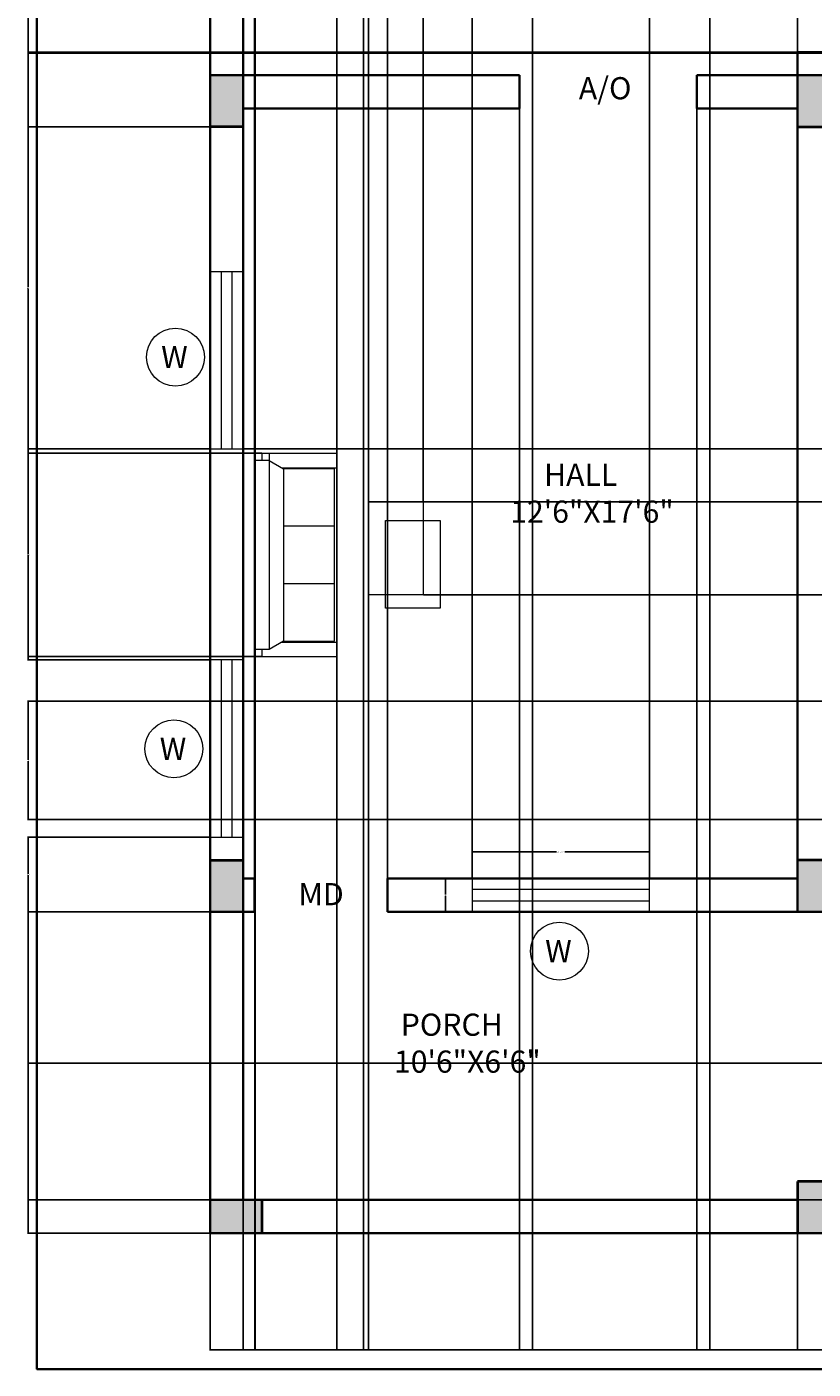
# Model space of a CAD drawing. Units: inches. Extents: x 2243 to 2668, y 14541 to 15226.
# Tile 1 of 5: x 2243 to 2456, y 14541 to 14904. Entities that reach past the tile are written whole.
import ezdxf

# ---------------------------------------------------------------- set-up
doc = ezdxf.new("R2010")
doc.units = ezdxf.units.IN
doc.header["$MEASUREMENT"] = 0
for name, color, linetype, lineweight in [('A-ANNO-DIMS', 2, 'Continuous', 18), ('A-ANNO-SYMB', 3, 'Continuous', 18), ('A-ANNO-TTLB', 7, 'Continuous', 35), ('A-AREA-IDEN', 7, 'Continuous', 18), ('A-COLS', 7, 'Continuous', 40), ('A-COLS-PATT', 7, 'Continuous', 13), ('A-FURN', 8, 'Continuous', 18), ('A-GLAZ', 4, 'Continuous', 18), ('A-WALL', 7, 'Continuous', 35)]:
    doc.layers.add(name, color=color, linetype=linetype, lineweight=lineweight)
doc.styles.get("Standard").update_dxf_attribs({"font": 'arial.ttf'})
doc.dimstyles.get("Standard").update_dxf_attribs({"dimtxt": 0.18, "dimasz": 0.18, "dimexe": 0.18, "dimexo": 0.0625, "dimgap": 0.09, "dimtad": 0, "dimtih": 1, "dimtoh": 1, "dimdec": 4, "dimzin": 0, "dimdsep": 46, "dimtxsty": 'Standard', "dimcen": 0.09, "dimadec": 0, "dimazin": 0, "dimtfac": 1, "dimtdec": 4, "dimtofl": 0, "dimtmove": 0, "dimatfit": 3, "dimfxl": 1, "dimtolj": 1, "dimtzin": 0, "dimarcsym": 0})

# ---------------------------------------------------------------- blocks, each defined once
blk = doc.blocks.new('WIN-48IN')
for p, q in [((0, 9), (0, 0)), ((48, 9), (0, 9)), ((48, 0), (48, 9)), ((48, 6), (0, 6)), ((0, 3), (48, 3)), ((0, 0), (48, 0))]:
    blk.add_line(p, q)
blk = doc.blocks.new('TAG-WINDOW-W')
blk.add_circle((7.84, 7.84), 7.84)
at = {"insert": (3.99, 10.84), "char_height": 6, "attachment_point": 1}
blk.add_mtext_dynamic_manual_height_columns('W', width=14.3449, gutter_width=30, heights=[0], dxfattribs=at)
blk = doc.blocks.new('*D7')
at = {"layer": 'A-ANNO-DIMS', "color": 0, "lineweight": -2, "transparency": 16777216}
for p, q in [((2363.89, 14673.7), (2363.89, 14681.02)), ((2364.07, 14680.84), (2386.77, 14680.84)), ((2411.71, 14680.84), (2389.01, 14680.84)), ((2411.89, 14673.7), (2411.89, 14681.02))]:
    blk.add_line(p, q, dxfattribs=at)
at = {"layer": 'A-ANNO-DIMS', "color": 0, "transparency": 16777216}
for points in [[(2364.07, 14680.87), (2364.07, 14680.81), (2363.89, 14680.84)], [(2411.71, 14680.87), (2411.71, 14680.81), (2411.89, 14680.84)]]:
    blk.add_solid(points, dxfattribs=at)
at = {"layer": 'Defpoints', "color": 0, "transparency": 16777216}
for p in [(2363.89, 14680.84), (2363.89, 14673.64), (2411.89, 14673.64)]:
    blk.add_point(p, dxfattribs=at)
at = {"layer": 'A-ANNO-DIMS', "color": 0, "transparency": 16777216, "insert": (2387.89, 14680.84), "char_height": 0.18, "attachment_point": 5}
blk.add_mtext('\\A1;WINDOW 48 TYP.', dxfattribs=at)
blk = doc.blocks.new('*D8')
at = {"layer": 'A-ANNO-DIMS', "color": 0, "lineweight": -2, "transparency": 16777216}
for p, q in [((2363.83, 14673.64), (2356.51, 14673.64)), ((2356.69, 14673.46), (2356.69, 14669.32)), ((2356.69, 14664.82), (2356.69, 14668.95)), ((2363.83, 14664.64), (2356.51, 14664.64))]:
    blk.add_line(p, q, dxfattribs=at)
at = {"layer": 'A-ANNO-DIMS', "color": 0, "transparency": 16777216}
for points in [[(2356.66, 14673.46), (2356.72, 14673.46), (2356.69, 14673.64)], [(2356.66, 14664.82), (2356.72, 14664.82), (2356.69, 14664.64)]]:
    blk.add_solid(points, dxfattribs=at)
at = {"layer": 'Defpoints', "color": 0, "transparency": 16777216}
for p in [(2363.89, 14673.64), (2356.69, 14664.64), (2363.89, 14664.64)]:
    blk.add_point(p, dxfattribs=at)
at = {"layer": 'A-ANNO-DIMS', "color": 0, "transparency": 16777216, "insert": (2356.69, 14669.14), "char_height": 0.18, "attachment_point": 5}
blk.add_mtext('\\A1;9 TYP.', dxfattribs=at)
blk = doc.blocks.new('*D19')
at = {"layer": 'A-ANNO-DIMS', "color": 0, "lineweight": -2, "transparency": 16777216}
for p, q in [((2292.96, 14577.57), (2292.96, 14545.86)), ((2451.96, 14577.57), (2451.96, 14545.86)), ((2293.14, 14546.04), (2372.18, 14546.04)), ((2451.78, 14546.04), (2372.74, 14546.04))]:
    blk.add_line(p, q, dxfattribs=at)
at = {"layer": 'A-ANNO-DIMS', "color": 0, "transparency": 16777216}
for points in [[(2293.14, 14546.07), (2293.14, 14546.01), (2292.96, 14546.04)], [(2451.78, 14546.07), (2451.78, 14546.01), (2451.96, 14546.04)]]:
    blk.add_solid(points, dxfattribs=at)
at = {"layer": 'Defpoints', "color": 0, "transparency": 16777216}
for p in [(2292.96, 14577.64), (2451.96, 14577.64), (2451.96, 14546.04)]:
    blk.add_point(p, dxfattribs=at)
at = {"layer": 'A-ANNO-DIMS', "color": 0, "transparency": 16777216, "insert": (2372.46, 14546.04), "char_height": 0.18, "attachment_point": 5}
blk.add_mtext('\\A1;159', dxfattribs=at)
blk = doc.blocks.new('*D20')
at = {"layer": 'A-ANNO-DIMS', "color": 0, "lineweight": -2, "transparency": 16777216}
for p, q in [((2451.96, 14577.57), (2451.96, 14545.86)), ((2604.96, 14577.57), (2604.96, 14545.86)), ((2452.14, 14546.04), (2528.18, 14546.04)), ((2604.78, 14546.04), (2528.74, 14546.04))]:
    blk.add_line(p, q, dxfattribs=at)
at = {"layer": 'A-ANNO-DIMS', "color": 0, "transparency": 16777216}
for points in [[(2452.14, 14546.07), (2452.14, 14546.01), (2451.96, 14546.04)], [(2604.78, 14546.07), (2604.78, 14546.01), (2604.96, 14546.04)]]:
    blk.add_solid(points, dxfattribs=at)
at = {"layer": 'Defpoints', "color": 0, "transparency": 16777216}
for p in [(2451.96, 14577.64), (2604.96, 14577.64), (2604.96, 14546.04)]:
    blk.add_point(p, dxfattribs=at)
at = {"layer": 'A-ANNO-DIMS', "color": 0, "transparency": 16777216, "insert": (2528.46, 14546.04), "char_height": 0.18, "attachment_point": 5}
blk.add_mtext('\\A1;153', dxfattribs=at)
blk = doc.blocks.new('*D21')
at = {"layer": 'A-ANNO-DIMS', "color": 0, "lineweight": -2, "transparency": 16777216}
for p, q in [((2292.9, 14664.64), (2243.57, 14664.64)), ((2243.75, 14664.46), (2243.75, 14621.32)), ((2243.75, 14577.82), (2243.75, 14620.95)), ((2292.9, 14577.64), (2243.57, 14577.64))]:
    blk.add_line(p, q, dxfattribs=at)
at = {"layer": 'A-ANNO-DIMS', "color": 0, "transparency": 16777216}
for points in [[(2243.72, 14664.46), (2243.78, 14664.46), (2243.75, 14664.64)], [(2243.72, 14577.82), (2243.78, 14577.82), (2243.75, 14577.64)]]:
    blk.add_solid(points, dxfattribs=at)
at = {"layer": 'Defpoints', "color": 0, "transparency": 16777216}
for p in [(2243.75, 14664.64), (2292.96, 14664.64), (2292.96, 14577.64)]:
    blk.add_point(p, dxfattribs=at)
at = {"layer": 'A-ANNO-DIMS', "color": 0, "transparency": 16777216, "insert": (2243.75, 14621.14), "char_height": 0.18, "attachment_point": 5}
blk.add_mtext('\\A1;87', dxfattribs=at)
blk = doc.blocks.new('*D22')
at = {"layer": 'A-ANNO-DIMS', "color": 0, "lineweight": -2, "transparency": 16777216}
for p, q in [((2292.9, 14684.86), (2243.57, 14684.86)), ((2243.75, 14684.68), (2243.75, 14674.93)), ((2243.75, 14664.82), (2243.75, 14674.57)), ((2292.9, 14664.64), (2243.57, 14664.64))]:
    blk.add_line(p, q, dxfattribs=at)
at = {"layer": 'A-ANNO-DIMS', "color": 0, "transparency": 16777216}
for points in [[(2243.72, 14684.68), (2243.78, 14684.68), (2243.75, 14684.86)], [(2243.72, 14664.82), (2243.78, 14664.82), (2243.75, 14664.64)]]:
    blk.add_solid(points, dxfattribs=at)
at = {"layer": 'Defpoints', "color": 0, "transparency": 16777216}
for p in [(2243.75, 14684.86), (2292.96, 14684.86), (2292.96, 14664.64)]:
    blk.add_point(p, dxfattribs=at)
at = {"layer": 'A-ANNO-DIMS', "color": 0, "transparency": 16777216, "insert": (2243.75, 14674.75), "char_height": 0.18, "attachment_point": 5}
blk.add_mtext('\\A1;20.225', dxfattribs=at)
blk = doc.blocks.new('*D23')
at = {"layer": 'A-ANNO-DIMS', "color": 0, "lineweight": -2, "transparency": 16777216}
for p, q in [((2292.9, 14789.95), (2243.57, 14789.95)), ((2243.75, 14789.77), (2243.75, 14761.59)), ((2243.75, 14733.04), (2243.75, 14761.22)), ((2292.9, 14732.86), (2243.57, 14732.86))]:
    blk.add_line(p, q, dxfattribs=at)
at = {"layer": 'A-ANNO-DIMS', "color": 0, "transparency": 16777216}
for points in [[(2243.72, 14789.77), (2243.78, 14789.77), (2243.75, 14789.95)], [(2243.72, 14733.04), (2243.78, 14733.04), (2243.75, 14732.86)]]:
    blk.add_solid(points, dxfattribs=at)
at = {"layer": 'Defpoints', "color": 0, "transparency": 16777216}
for p in [(2243.75, 14789.95), (2292.96, 14789.95), (2292.96, 14732.86)]:
    blk.add_point(p, dxfattribs=at)
at = {"layer": 'A-ANNO-DIMS', "color": 0, "transparency": 16777216, "insert": (2243.75, 14761.41), "char_height": 0.18, "attachment_point": 5}
blk.add_mtext('\\A1;57.09', dxfattribs=at)
blk = doc.blocks.new('*D24')
at = {"layer": 'A-ANNO-DIMS', "color": 0, "lineweight": -2, "transparency": 16777216}
for p, q in [((2292.9, 14877.14), (2243.57, 14877.14)), ((2243.75, 14876.96), (2243.75, 14833.73)), ((2243.75, 14790.13), (2243.75, 14833.36)), ((2292.9, 14789.95), (2243.57, 14789.95))]:
    blk.add_line(p, q, dxfattribs=at)
at = {"layer": 'A-ANNO-DIMS', "color": 0, "transparency": 16777216}
for points in [[(2243.72, 14876.96), (2243.78, 14876.96), (2243.75, 14877.14)], [(2243.72, 14790.13), (2243.78, 14790.13), (2243.75, 14789.95)]]:
    blk.add_solid(points, dxfattribs=at)
at = {"layer": 'Defpoints', "color": 0, "transparency": 16777216}
for p in [(2243.75, 14877.14), (2292.96, 14877.14), (2292.96, 14789.95)]:
    blk.add_point(p, dxfattribs=at)
at = {"layer": 'A-ANNO-DIMS', "color": 0, "transparency": 16777216, "insert": (2243.75, 14833.54), "char_height": 0.18, "attachment_point": 5}
blk.add_mtext('\\A1;87.19', dxfattribs=at)
blk = doc.blocks.new('*D25')
at = {"layer": 'A-ANNO-DIMS', "color": 0, "lineweight": -2, "transparency": 16777216}
for p, q in [((2292.9, 14940.64), (2243.57, 14940.64)), ((2243.75, 14940.46), (2243.75, 14909.07)), ((2243.75, 14877.32), (2243.75, 14908.71)), ((2292.9, 14877.14), (2243.57, 14877.14))]:
    blk.add_line(p, q, dxfattribs=at)
at = {"layer": 'A-ANNO-DIMS', "color": 0, "transparency": 16777216}
for points in [[(2243.72, 14940.46), (2243.78, 14940.46), (2243.75, 14940.64)], [(2243.72, 14877.32), (2243.78, 14877.32), (2243.75, 14877.14)]]:
    blk.add_solid(points, dxfattribs=at)
at = {"layer": 'Defpoints', "color": 0, "transparency": 16777216}
for p in [(2243.75, 14940.64), (2292.96, 14940.64), (2292.96, 14877.14)]:
    blk.add_point(p, dxfattribs=at)
at = {"layer": 'A-ANNO-DIMS', "color": 0, "transparency": 16777216, "insert": (2243.75, 14908.89), "char_height": 0.18, "attachment_point": 5}
blk.add_mtext('\\A1;63.5', dxfattribs=at)
blk = doc.blocks.new('*D32')
at = {"layer": 'A-ANNO-DIMS', "color": 0, "lineweight": -2, "transparency": 16777216}
for p, q in [((2301.96, 14673.7), (2301.96, 15225.04)), ((2302.14, 15224.86), (2303.31, 15224.86)), ((2304.78, 15224.86), (2303.61, 15224.86)), ((2304.96, 14673.7), (2304.96, 15225.04))]:
    blk.add_line(p, q, dxfattribs=at)
at = {"layer": 'A-ANNO-DIMS', "color": 0, "transparency": 16777216}
for points in [[(2302.14, 15224.89), (2302.14, 15224.83), (2301.96, 15224.86)], [(2304.78, 15224.89), (2304.78, 15224.83), (2304.96, 15224.86)]]:
    blk.add_solid(points, dxfattribs=at)
at = {"layer": 'Defpoints', "color": 0, "transparency": 16777216}
for p in [(2304.96, 15224.86), (2301.96, 14673.64), (2304.96, 14673.64)]:
    blk.add_point(p, dxfattribs=at)
at = {"layer": 'A-ANNO-DIMS', "color": 0, "transparency": 16777216, "insert": (2303.46, 15224.86), "char_height": 0.18, "attachment_point": 5}
blk.add_mtext('\\A1;3', dxfattribs=at)
blk = doc.blocks.new('*D33')
at = {"layer": 'A-ANNO-DIMS', "color": 0, "lineweight": -2, "transparency": 16777216}
for p, q in [((2304.96, 14673.7), (2304.96, 15225.04)), ((2305.14, 15224.86), (2322.74, 15224.86)), ((2340.78, 15224.86), (2323.18, 15224.86)), ((2340.96, 14673.7), (2340.96, 15225.04))]:
    blk.add_line(p, q, dxfattribs=at)
at = {"layer": 'A-ANNO-DIMS', "color": 0, "transparency": 16777216}
for points in [[(2305.14, 15224.89), (2305.14, 15224.83), (2304.96, 15224.86)], [(2340.78, 15224.89), (2340.78, 15224.83), (2340.96, 15224.86)]]:
    blk.add_solid(points, dxfattribs=at)
at = {"layer": 'Defpoints', "color": 0, "transparency": 16777216}
for p in [(2340.96, 15224.86), (2304.96, 14673.64), (2340.96, 14673.64)]:
    blk.add_point(p, dxfattribs=at)
at = {"layer": 'A-ANNO-DIMS', "color": 0, "transparency": 16777216, "insert": (2322.96, 15224.86), "char_height": 0.18, "attachment_point": 5}
blk.add_mtext('\\A1;36', dxfattribs=at)
blk = doc.blocks.new('*D34')
at = {"layer": 'A-ANNO-DIMS', "color": 0, "lineweight": -2, "transparency": 16777216}
for p, q in [((2340.96, 14673.7), (2340.96, 15225.04)), ((2341.14, 15224.86), (2352.03, 15224.86)), ((2363.71, 15224.86), (2352.82, 15224.86)), ((2363.89, 14673.7), (2363.89, 15225.04))]:
    blk.add_line(p, q, dxfattribs=at)
at = {"layer": 'A-ANNO-DIMS', "color": 0, "transparency": 16777216}
for points in [[(2341.14, 15224.89), (2341.14, 15224.83), (2340.96, 15224.86)], [(2363.71, 15224.89), (2363.71, 15224.83), (2363.89, 15224.86)]]:
    blk.add_solid(points, dxfattribs=at)
at = {"layer": 'Defpoints', "color": 0, "transparency": 16777216}
for p in [(2363.89, 15224.86), (2340.96, 14673.64), (2363.89, 14673.64)]:
    blk.add_point(p, dxfattribs=at)
at = {"layer": 'A-ANNO-DIMS', "color": 0, "transparency": 16777216, "insert": (2352.43, 15224.86), "char_height": 0.18, "attachment_point": 5}
blk.add_mtext('\\A1;22.93', dxfattribs=at)
blk = doc.blocks.new('*D35')
at = {"layer": 'A-ANNO-DIMS', "color": 0, "lineweight": -2, "transparency": 16777216}
for p, q in [((2411.89, 14673.7), (2411.89, 15225.04)), ((2412.07, 15224.86), (2431.53, 15224.86)), ((2451.78, 15224.86), (2432.32, 15224.86)), ((2451.96, 14673.7), (2451.96, 15225.04))]:
    blk.add_line(p, q, dxfattribs=at)
at = {"layer": 'A-ANNO-DIMS', "color": 0, "transparency": 16777216}
for points in [[(2412.07, 15224.89), (2412.07, 15224.83), (2411.89, 15224.86)], [(2451.78, 15224.89), (2451.78, 15224.83), (2451.96, 15224.86)]]:
    blk.add_solid(points, dxfattribs=at)
at = {"layer": 'Defpoints', "color": 0, "transparency": 16777216}
for p in [(2451.96, 15224.86), (2411.89, 14673.64), (2451.96, 14673.64)]:
    blk.add_point(p, dxfattribs=at)
at = {"layer": 'A-ANNO-DIMS', "color": 0, "transparency": 16777216, "insert": (2431.93, 15224.86), "char_height": 0.18, "attachment_point": 5}
blk.add_mtext('\\A1;40.07', dxfattribs=at)
blk = doc.blocks.new('*D38')
at = {"layer": 'A-ANNO-DIMS', "color": 0, "lineweight": -2, "transparency": 16777216}
for p, q in [((2463.9, 14623.64), (2243.57, 14623.64)), ((2243.75, 14623.46), (2243.75, 14605.32)), ((2243.75, 14586.82), (2243.75, 14604.95)), ((2463.9, 14586.64), (2243.57, 14586.64))]:
    blk.add_line(p, q, dxfattribs=at)
at = {"layer": 'A-ANNO-DIMS', "color": 0, "transparency": 16777216}
for points in [[(2243.72, 14623.46), (2243.78, 14623.46), (2243.75, 14623.64)], [(2243.72, 14586.82), (2243.78, 14586.82), (2243.75, 14586.64)]]:
    blk.add_solid(points, dxfattribs=at)
at = {"layer": 'Defpoints', "color": 0, "transparency": 16777216}
for p in [(2243.75, 14623.64), (2463.96, 14623.64), (2463.96, 14586.64)]:
    blk.add_point(p, dxfattribs=at)
at = {"layer": 'A-ANNO-DIMS', "color": 0, "transparency": 16777216, "insert": (2243.75, 14605.14), "char_height": 0.18, "attachment_point": 5}
blk.add_mtext('\\A1;37', dxfattribs=at)
blk = doc.blocks.new('*D42')
at = {"layer": 'A-ANNO-DIMS', "color": 0, "lineweight": -2, "transparency": 16777216}
for p, q in [((2380.28, 15014.07), (2380.28, 14545.86)), ((2428.28, 15014.07), (2428.28, 14545.86)), ((2380.46, 14546.04), (2404.06, 14546.04)), ((2428.1, 14546.04), (2404.5, 14546.04))]:
    blk.add_line(p, q, dxfattribs=at)
at = {"layer": 'A-ANNO-DIMS', "color": 0, "transparency": 16777216}
for points in [[(2380.46, 14546.07), (2380.46, 14546.01), (2380.28, 14546.04)], [(2428.1, 14546.07), (2428.1, 14546.01), (2428.28, 14546.04)]]:
    blk.add_solid(points, dxfattribs=at)
at = {"layer": 'Defpoints', "color": 0, "transparency": 16777216}
for p in [(2380.28, 15014.14), (2428.28, 15014.14), (2428.28, 14546.04)]:
    blk.add_point(p, dxfattribs=at)
at = {"layer": 'A-ANNO-DIMS', "color": 0, "transparency": 16777216, "insert": (2404.28, 14546.04), "char_height": 0.18, "attachment_point": 5}
blk.add_mtext('\\A1;48', dxfattribs=at)
blk = doc.blocks.new('*D43')
at = {"layer": 'A-ANNO-DIMS', "color": 0, "lineweight": -2, "transparency": 16777216}
for p, q in [((2301.96, 15023.07), (2301.96, 14545.86)), ((2334.46, 15023.07), (2334.46, 14545.86)), ((2302.14, 14546.04), (2317.89, 14546.04)), ((2334.28, 14546.04), (2318.54, 14546.04))]:
    blk.add_line(p, q, dxfattribs=at)
at = {"layer": 'A-ANNO-DIMS', "color": 0, "transparency": 16777216}
for points in [[(2302.14, 14546.07), (2302.14, 14546.01), (2301.96, 14546.04)], [(2334.28, 14546.07), (2334.28, 14546.01), (2334.46, 14546.04)]]:
    blk.add_solid(points, dxfattribs=at)
at = {"layer": 'Defpoints', "color": 0, "transparency": 16777216}
for p in [(2301.96, 15023.14), (2334.46, 15023.14), (2334.46, 14546.04)]:
    blk.add_point(p, dxfattribs=at)
at = {"layer": 'A-ANNO-DIMS', "color": 0, "transparency": 16777216, "insert": (2318.21, 14546.04), "char_height": 0.18, "attachment_point": 5}
blk.add_mtext('\\A1;32.5', dxfattribs=at)
blk = doc.blocks.new('*D47')
at = {"layer": 'A-ANNO-DIMS', "color": 0, "lineweight": -2, "transparency": 16777216}
for p, q in [((2376.7, 14882.07), (2376.7, 14545.86)), ((2424.7, 14882.07), (2424.7, 14545.86)), ((2376.88, 14546.04), (2400.48, 14546.04)), ((2424.52, 14546.04), (2400.92, 14546.04))]:
    blk.add_line(p, q, dxfattribs=at)
at = {"layer": 'A-ANNO-DIMS', "color": 0, "transparency": 16777216}
for points in [[(2376.88, 14546.07), (2376.88, 14546.01), (2376.7, 14546.04)], [(2424.52, 14546.07), (2424.52, 14546.01), (2424.7, 14546.04)]]:
    blk.add_solid(points, dxfattribs=at)
at = {"layer": 'Defpoints', "color": 0, "transparency": 16777216}
for p in [(2376.7, 14882.14), (2424.7, 14882.14), (2424.7, 14546.04)]:
    blk.add_point(p, dxfattribs=at)
at = {"layer": 'A-ANNO-DIMS', "color": 0, "transparency": 16777216, "insert": (2400.7, 14546.04), "char_height": 0.18, "attachment_point": 5}
blk.add_mtext('\\A1;48', dxfattribs=at)
blk = doc.blocks.new('*D50')
at = {"layer": 'A-ANNO-DIMS', "color": 0, "lineweight": -2, "transparency": 16777216}
for p, q in [((2513.4, 14721.64), (2243.57, 14721.64)), ((2243.75, 14721.46), (2243.75, 14705.82)), ((2243.75, 14689.82), (2243.75, 14705.45)), ((2513.4, 14689.64), (2243.57, 14689.64))]:
    blk.add_line(p, q, dxfattribs=at)
at = {"layer": 'A-ANNO-DIMS', "color": 0, "transparency": 16777216}
for points in [[(2243.72, 14721.46), (2243.78, 14721.46), (2243.75, 14721.64)], [(2243.72, 14689.82), (2243.78, 14689.82), (2243.75, 14689.64)]]:
    blk.add_solid(points, dxfattribs=at)
at = {"layer": 'Defpoints', "color": 0, "transparency": 16777216}
for p in [(2243.75, 14721.64), (2513.46, 14721.64), (2513.46, 14689.64)]:
    blk.add_point(p, dxfattribs=at)
at = {"layer": 'A-ANNO-DIMS', "color": 0, "transparency": 16777216, "insert": (2243.75, 14705.64), "char_height": 0.18, "attachment_point": 5}
blk.add_mtext('\\A1;32', dxfattribs=at)
blk = doc.blocks.new('*D51')
at = {"layer": 'A-ANNO-DIMS', "color": 0, "lineweight": -2, "transparency": 16777216}
for p, q in [((2531.4, 14929.14), (2243.57, 14929.14)), ((2243.75, 14928.96), (2243.75, 14913.32)), ((2243.75, 14897.32), (2243.75, 14912.95)), ((2531.4, 14897.14), (2243.57, 14897.14))]:
    blk.add_line(p, q, dxfattribs=at)
at = {"layer": 'A-ANNO-DIMS', "color": 0, "transparency": 16777216}
for points in [[(2243.72, 14928.96), (2243.78, 14928.96), (2243.75, 14929.14)], [(2243.72, 14897.32), (2243.78, 14897.32), (2243.75, 14897.14)]]:
    blk.add_solid(points, dxfattribs=at)
at = {"layer": 'Defpoints', "color": 0, "transparency": 16777216}
for p in [(2243.75, 14929.14), (2531.46, 14929.14), (2531.46, 14897.14)]:
    blk.add_point(p, dxfattribs=at)
at = {"layer": 'A-ANNO-DIMS', "color": 0, "transparency": 16777216, "insert": (2243.75, 14913.14), "char_height": 0.18, "attachment_point": 5}
blk.add_mtext('\\A1;32', dxfattribs=at)
blk = doc.blocks.new('*D54')
at = {"layer": 'A-ANNO-DIMS', "color": 0, "lineweight": -2, "transparency": 16777216}
for p, q in [((2451.9, 14957.21), (2243.57, 14957.21)), ((2243.75, 14957.03), (2243.75, 14927.48)), ((2243.75, 14897.56), (2243.75, 14927.11)), ((2451.9, 14897.38), (2243.57, 14897.38))]:
    blk.add_line(p, q, dxfattribs=at)
at = {"layer": 'A-ANNO-DIMS', "color": 0, "transparency": 16777216}
for points in [[(2243.72, 14957.03), (2243.78, 14957.03), (2243.75, 14957.21)], [(2243.72, 14897.56), (2243.78, 14897.56), (2243.75, 14897.38)]]:
    blk.add_solid(points, dxfattribs=at)
at = {"layer": 'Defpoints', "color": 0, "transparency": 16777216}
for p in [(2243.75, 14957.21), (2451.96, 14957.21), (2451.96, 14897.38)]:
    blk.add_point(p, dxfattribs=at)
at = {"layer": 'A-ANNO-DIMS', "color": 0, "transparency": 16777216, "insert": (2243.75, 14927.3), "char_height": 0.18, "attachment_point": 5}
blk.add_mtext('\\A1;59.83', dxfattribs=at)
blk = doc.blocks.new('*D56')
at = {"layer": 'A-ANNO-DIMS', "color": 0, "lineweight": -2, "transparency": 16777216}
for p, q in [((2305.04, 14786.87), (2305.04, 15225.04)), ((2305.22, 15224.86), (2315.76, 15224.86)), ((2327.09, 15224.86), (2316.55, 15224.86)), ((2327.27, 14788.83), (2327.27, 15225.04))]:
    blk.add_line(p, q, dxfattribs=at)
at = {"layer": 'A-ANNO-DIMS', "color": 0, "transparency": 16777216}
for points in [[(2305.22, 15224.89), (2305.22, 15224.83), (2305.04, 15224.86)], [(2327.09, 15224.89), (2327.09, 15224.83), (2327.27, 15224.86)]]:
    blk.add_solid(points, dxfattribs=at)
at = {"layer": 'Defpoints', "color": 0, "transparency": 16777216}
for p in [(2327.27, 15224.86), (2327.27, 14788.77), (2305.04, 14786.81)]:
    blk.add_point(p, dxfattribs=at)
at = {"layer": 'A-ANNO-DIMS', "color": 0, "transparency": 16777216, "insert": (2316.15, 15224.86), "char_height": 0.18, "attachment_point": 5}
blk.add_mtext('\\A1;22.23', dxfattribs=at)
blk = doc.blocks.new('*D57')
at = {"layer": 'A-ANNO-DIMS', "color": 0, "lineweight": -2, "transparency": 16777216}
for p, q in [((2306.94, 14788.77), (2243.57, 14788.77)), ((2243.75, 14788.59), (2243.75, 14761.43)), ((2243.75, 14733.9), (2243.75, 14761.06)), ((2306.94, 14733.72), (2243.57, 14733.72))]:
    blk.add_line(p, q, dxfattribs=at)
at = {"layer": 'A-ANNO-DIMS', "color": 0, "transparency": 16777216}
for points in [[(2243.72, 14788.59), (2243.78, 14788.59), (2243.75, 14788.77)], [(2243.72, 14733.9), (2243.78, 14733.9), (2243.75, 14733.72)]]:
    blk.add_solid(points, dxfattribs=at)
at = {"layer": 'Defpoints', "color": 0, "transparency": 16777216}
for p in [(2307, 14788.77), (2243.75, 14733.72), (2307, 14733.72)]:
    blk.add_point(p, dxfattribs=at)
at = {"layer": 'A-ANNO-DIMS', "color": 0, "transparency": 16777216, "insert": (2243.75, 14761.24), "char_height": 0.18, "attachment_point": 5}
blk.add_mtext('\\A1;55.04', dxfattribs=at)
blk = doc.blocks.new('*D58')
at = {"layer": 'A-ANNO-DIMS', "color": 0, "lineweight": -2, "transparency": 16777216}
for p, q in [((2327.27, 14788.7), (2327.27, 14545.86)), ((2335.83, 14775.57), (2335.83, 14545.86)), ((2327.45, 14546.04), (2331.15, 14546.04)), ((2335.65, 14546.04), (2331.94, 14546.04))]:
    blk.add_line(p, q, dxfattribs=at)
at = {"layer": 'A-ANNO-DIMS', "color": 0, "transparency": 16777216}
for points in [[(2327.45, 14546.07), (2327.45, 14546.01), (2327.27, 14546.04)], [(2335.65, 14546.07), (2335.65, 14546.01), (2335.83, 14546.04)]]:
    blk.add_solid(points, dxfattribs=at)
at = {"layer": 'Defpoints', "color": 0, "transparency": 16777216}
for p in [(2327.27, 14788.77), (2335.83, 14775.64), (2335.83, 14546.04)]:
    blk.add_point(p, dxfattribs=at)
at = {"layer": 'A-ANNO-DIMS', "color": 0, "transparency": 16777216, "insert": (2331.55, 14546.04), "char_height": 0.18, "attachment_point": 5}
blk.add_mtext('\\A1;8.562', dxfattribs=at)
blk = doc.blocks.new('*D59')
at = {"layer": 'A-ANNO-DIMS', "color": 0, "lineweight": -2, "transparency": 16777216}
for p, q in [((2335.83, 14775.7), (2335.83, 15225.04)), ((2336.01, 15224.86), (2342.78, 15224.86)), ((2350.47, 15224.86), (2343.69, 15224.86)), ((2350.65, 14775.7), (2350.65, 15225.04))]:
    blk.add_line(p, q, dxfattribs=at)
at = {"layer": 'A-ANNO-DIMS', "color": 0, "transparency": 16777216}
for points in [[(2336.01, 15224.89), (2336.01, 15224.83), (2335.83, 15224.86)], [(2350.47, 15224.89), (2350.47, 15224.83), (2350.65, 15224.86)]]:
    blk.add_solid(points, dxfattribs=at)
at = {"layer": 'Defpoints', "color": 0, "transparency": 16777216}
for p in [(2350.65, 15224.86), (2335.83, 14775.64), (2350.65, 14775.64)]:
    blk.add_point(p, dxfattribs=at)
at = {"layer": 'A-ANNO-DIMS', "color": 0, "transparency": 16777216, "insert": (2343.24, 15224.86), "char_height": 0.18, "attachment_point": 5}
blk.add_mtext('\\A1;14.818', dxfattribs=at)
blk = doc.blocks.new('*D60')
at = {"layer": 'A-ANNO-DIMS', "color": 0, "lineweight": -2, "transparency": 16777216}
for p, q in [((2350.71, 14775.64), (2653.58, 14775.64)), ((2653.4, 14775.46), (2653.4, 14763.21)), ((2653.4, 14750.6), (2653.4, 14762.85)), ((2350.71, 14750.42), (2653.58, 14750.42))]:
    blk.add_line(p, q, dxfattribs=at)
at = {"layer": 'A-ANNO-DIMS', "color": 0, "transparency": 16777216}
for points in [[(2653.37, 14775.46), (2653.43, 14775.46), (2653.4, 14775.64)], [(2653.37, 14750.6), (2653.43, 14750.6), (2653.4, 14750.42)]]:
    blk.add_solid(points, dxfattribs=at)
at = {"layer": 'Defpoints', "color": 0, "transparency": 16777216}
for p in [(2350.65, 14775.64), (2653.4, 14775.64), (2350.65, 14750.42)]:
    blk.add_point(p, dxfattribs=at)
at = {"layer": 'A-ANNO-DIMS', "color": 0, "transparency": 16777216, "insert": (2653.4, 14763.03), "char_height": 0.18, "attachment_point": 5}
blk.add_mtext('\\A1;25.22', dxfattribs=at)
blk = doc.blocks.new('*D61')
at = {"layer": 'A-ANNO-DIMS', "color": 0, "lineweight": -2, "transparency": 16777216}
for p, q in [((2301.96, 15023.07), (2301.96, 14545.86)), ((2380.28, 15014.07), (2380.28, 14545.86)), ((2302.14, 14546.04), (2340.73, 14546.04)), ((2380.1, 14546.04), (2341.51, 14546.04))]:
    blk.add_line(p, q, dxfattribs=at)
at = {"layer": 'A-ANNO-DIMS', "color": 0, "transparency": 16777216}
for points in [[(2302.14, 14546.07), (2302.14, 14546.01), (2301.96, 14546.04)], [(2380.1, 14546.07), (2380.1, 14546.01), (2380.28, 14546.04)]]:
    blk.add_solid(points, dxfattribs=at)
at = {"layer": 'Defpoints', "color": 0, "transparency": 16777216}
for p in [(2301.96, 15023.14), (2380.28, 15014.14), (2380.28, 14546.04)]:
    blk.add_point(p, dxfattribs=at)
at = {"layer": 'A-ANNO-DIMS', "color": 0, "transparency": 16777216, "insert": (2341.12, 14546.04), "char_height": 0.18, "attachment_point": 5}
blk.add_mtext('\\A1;78.32', dxfattribs=at)
blk = doc.blocks.new('*D62')
at = {"layer": 'A-ANNO-DIMS', "color": 0, "lineweight": -2, "transparency": 16777216}
for p, q in [((2301.96, 14882.07), (2301.96, 14545.86)), ((2376.7, 14882.07), (2376.7, 14545.86)), ((2302.14, 14546.04), (2338.94, 14546.04)), ((2376.52, 14546.04), (2339.72, 14546.04))]:
    blk.add_line(p, q, dxfattribs=at)
at = {"layer": 'A-ANNO-DIMS', "color": 0, "transparency": 16777216}
for points in [[(2302.14, 14546.07), (2302.14, 14546.01), (2301.96, 14546.04)], [(2376.52, 14546.07), (2376.52, 14546.01), (2376.7, 14546.04)]]:
    blk.add_solid(points, dxfattribs=at)
at = {"layer": 'Defpoints', "color": 0, "transparency": 16777216}
for p in [(2301.96, 14882.14), (2376.7, 14882.14), (2376.7, 14546.04)]:
    blk.add_point(p, dxfattribs=at)
at = {"layer": 'A-ANNO-DIMS', "color": 0, "transparency": 16777216, "insert": (2339.33, 14546.04), "char_height": 0.18, "attachment_point": 5}
blk.add_mtext('\\A1;74.74', dxfattribs=at)
blk = doc.blocks.new('*D63')
at = {"layer": 'A-ANNO-DIMS', "color": 0, "lineweight": -2, "transparency": 16777216}
for p, q in [((2305.04, 14735.62), (2305.04, 14545.86)), ((2301.96, 14732.8), (2301.96, 14545.86)), ((2302.14, 14546.04), (2303.1, 14546.04)), ((2304.86, 14546.04), (2303.89, 14546.04))]:
    blk.add_line(p, q, dxfattribs=at)
at = {"layer": 'A-ANNO-DIMS', "color": 0, "transparency": 16777216}
for points in [[(2302.14, 14546.07), (2302.14, 14546.01), (2301.96, 14546.04)], [(2304.86, 14546.07), (2304.86, 14546.01), (2305.04, 14546.04)]]:
    blk.add_solid(points, dxfattribs=at)
at = {"layer": 'Defpoints', "color": 0, "transparency": 16777216}
for p in [(2305.04, 14735.68), (2301.96, 14732.86), (2305.04, 14546.04)]:
    blk.add_point(p, dxfattribs=at)
at = {"layer": 'A-ANNO-DIMS', "color": 0, "transparency": 16777216, "insert": (2303.5, 14546.04), "char_height": 0.18, "attachment_point": 5}
blk.add_mtext('\\A1;3.077', dxfattribs=at)
blk = doc.blocks.new('*D64')
at = {"layer": 'A-ANNO-DIMS', "color": 0, "lineweight": -2, "transparency": 16777216}
for p, q in [((2302.02, 14789.95), (2653.58, 14789.95)), ((2653.4, 14789.77), (2653.4, 14782.98)), ((2653.4, 14775.82), (2653.4, 14782.61)), ((2335.89, 14775.64), (2653.58, 14775.64))]:
    blk.add_line(p, q, dxfattribs=at)
at = {"layer": 'A-ANNO-DIMS', "color": 0, "transparency": 16777216}
for points in [[(2653.37, 14789.77), (2653.43, 14789.77), (2653.4, 14789.95)], [(2653.37, 14775.82), (2653.43, 14775.82), (2653.4, 14775.64)]]:
    blk.add_solid(points, dxfattribs=at)
at = {"layer": 'Defpoints', "color": 0, "transparency": 16777216}
for p in [(2301.96, 14789.95), (2335.83, 14775.64), (2653.4, 14775.64)]:
    blk.add_point(p, dxfattribs=at)
at = {"layer": 'A-ANNO-DIMS', "color": 0, "transparency": 16777216, "insert": (2653.4, 14782.79), "char_height": 0.18, "attachment_point": 5}
blk.add_mtext('\\A1;14.312', dxfattribs=at)
blk = doc.blocks.new('*D65')
at = {"layer": 'A-ANNO-DIMS', "color": 0, "lineweight": -2, "transparency": 16777216}
for p, q in [((2305.17, 15053.26), (2305.17, 14545.86)), ((2301.96, 15035.22), (2301.96, 14545.86)), ((2302.14, 14546.04), (2303.26, 14546.04)), ((2304.99, 14546.04), (2303.87, 14546.04))]:
    blk.add_line(p, q, dxfattribs=at)
at = {"layer": 'A-ANNO-DIMS', "color": 0, "transparency": 16777216}
for points in [[(2302.14, 14546.07), (2302.14, 14546.01), (2301.96, 14546.04)], [(2304.99, 14546.07), (2304.99, 14546.01), (2305.17, 14546.04)]]:
    blk.add_solid(points, dxfattribs=at)
at = {"layer": 'Defpoints', "color": 0, "transparency": 16777216}
for p in [(2305.17, 15053.32), (2301.96, 15035.28), (2305.17, 14546.04)]:
    blk.add_point(p, dxfattribs=at)
at = {"layer": 'A-ANNO-DIMS', "color": 0, "transparency": 16777216, "insert": (2303.56, 14546.04), "char_height": 0.18, "attachment_point": 5}
blk.add_mtext('\\A1;3.21', dxfattribs=at)

msp = doc.modelspace()

# ---------------------------------------------------------------- hatches: boundary and pattern name
at = {"layer": 'A-COLS-PATT'}
h = msp.add_hatch(color=256, dxfattribs=at)
h.dxf.hatch_style = 1
h.paths.add_polyline_path([(2301.96, 15176.1368), (2292.96, 15176.1368), (2292.96, 15162.1368), (2301.96, 15162.1368)])
h.paths.add_polyline_path([(2460.96, 15176.1368), (2451.96, 15176.1368), (2451.96, 15162.1368), (2460.96, 15162.1368)])
h.paths.add_polyline_path([(2604.96, 15176.1368), (2595.96, 15176.1368), (2595.96, 15162.1368), (2604.96, 15162.1368)])
h.paths.add_polyline_path([(2301.96, 15028.1368), (2292.96, 15028.1368), (2292.96, 15014.1368), (2301.96, 15014.1368)])
h.paths.add_polyline_path([(2460.96, 15028.1368), (2451.96, 15028.1368), (2451.96, 15014.1368), (2460.96, 15014.1368)])
h.paths.add_polyline_path([(2604.96, 15027.8868), (2595.96, 15027.8868), (2595.96, 15013.8868), (2604.96, 15013.8868)])
h.paths.add_polyline_path([(2301.96, 14891.1368), (2292.96, 14891.1368), (2292.96, 14877.1368), (2301.96, 14877.1368)])
h.paths.add_polyline_path([(2460.96, 14891.1368), (2451.96, 14891.1368), (2451.96, 14877.1368), (2460.96, 14877.1368)])
h.paths.add_polyline_path([(2604.96, 14891.1368), (2595.96, 14891.1368), (2595.96, 14877.1368), (2604.96, 14877.1368)])
h.paths.add_polyline_path([(2301.96, 14678.6368), (2292.96, 14678.6368), (2292.96, 14664.6368), (2301.96, 14664.6368)])
h.paths.add_polyline_path([(2460.96, 14678.6368), (2451.96, 14678.6368), (2451.96, 14664.6368), (2460.96, 14664.6368)])
h.paths.add_polyline_path([(2604.96, 14678.6368), (2595.96, 14678.6368), (2595.96, 14664.6368), (2604.96, 14664.6368)])
h.paths.add_polyline_path([(2604.96, 14591.6368), (2595.96, 14591.6368), (2595.96, 14577.6368), (2604.96, 14577.6368)])
h.paths.add_polyline_path([(2460.96, 14591.6368), (2451.96, 14591.6368), (2451.96, 14577.6368), (2460.96, 14577.6368)])
h.paths.add_polyline_path([(2306.96, 14586.6368), (2292.96, 14586.6368), (2292.96, 14577.6368), (2306.96, 14577.6368)])

# ---------------------------------------------------------------- linework, layer by layer
at = {"layer": 'A-ANNO-TTLB'}
msp.add_lwpolyline([(2246.1122, 15225.9536), (2667.5226, 15225.9536), (2667.5226, 14540.814), (2246.1122, 14540.814)], close=True, dxfattribs=at)
at = {"layer": 'A-COLS'}
for p, q in [((2301.96, 14877.1368), (2292.96, 14877.1368)), ((2451.96, 14877.1368), (2460.96, 14877.1368)), ((2292.96, 14678.6368), (2301.96, 14678.6368)), ((2460.96, 14678.6368), (2451.96, 14678.6368)), ((2460.96, 14591.6368), (2451.96, 14591.6368)), ((2451.96, 14591.6368), (2451.96, 14577.6368)), ((2306.96, 14586.6368), (2306.96, 14577.6368))]:
    msp.add_line(p, q, dxfattribs=at)
at = {"layer": 'A-FURN'}
for p, q in [((2306.9985, 14788.7668), (2327.2661, 14788.7668)), ((2306.9985, 14788.7668), (2306.9985, 14786.8054)), ((2308.9599, 14788.7668), (2308.9599, 14735.6842)), ((2327.2661, 14784.844), (2327.2661, 14788.7668)), ((2305.0371, 14786.8054), (2305.0371, 14735.6842)), ((2308.9599, 14786.8054), (2305.0371, 14786.8054)), ((2308.9599, 14786.8054), (2312.8826, 14784.5989)), ((2312.5809, 14784.844), (2327.2661, 14784.844)), ((2326.6123, 14784.5962), (2312.8826, 14784.5962)), ((2326.6123, 14769.0277), (2312.8826, 14769.0277)), ((2326.6123, 14753.4592), (2312.8826, 14753.4592)), ((2312.8826, 14737.8908), (2308.9599, 14735.6842)), ((2312.3222, 14737.6456), (2327.2661, 14737.6456)), ((2327.2661, 14737.6456), (2327.2661, 14733.7228)), ((2308.9599, 14735.6842), (2305.0371, 14735.6842)), ((2306.9985, 14735.6842), (2306.9985, 14733.7228)), ((2306.9985, 14733.7228), (2327.2661, 14733.7228))]:
    msp.add_line(p, q, dxfattribs=at)
msp.add_lwpolyline([(2312.8826, 14784.5989), (2312.8826, 14737.8908), (2326.6123, 14737.8908), (2326.6123, 14784.5962)], dxfattribs=at)
for points in [[(2335.8284, 14775.637), (2350.6465, 14775.637), (2350.6465, 14750.4188), (2335.8284, 14750.4188)], [(2340.4738, 14770.5816), (2355.2919, 14770.5816), (2355.2919, 14746.833), (2340.4738, 14746.833)]]:
    msp.add_lwpolyline(points, close=True, dxfattribs=at)
at = {"layer": 'A-WALL'}
for p, q in [((2292.96, 15176.1368), (2292.96, 14577.6368)), ((2301.96, 15176.1368), (2301.96, 14586.6368)), ((2460.96, 14897.3823), (2451.96, 14897.3823)), ((2451.96, 14897.3823), (2451.96, 14664.6368)), ((2292.96, 14891.1368), (2376.7001, 14891.1368)), ((2376.7001, 14882.1368), (2376.7001, 14891.1368)), ((2424.7001, 14891.1368), (2424.7001, 14882.1368)), ((2424.7001, 14891.1368), (2463.96, 14891.1368)), ((2301.96, 14882.1368), (2376.7001, 14882.1368)), ((2424.7001, 14882.1368), (2451.96, 14882.1368)), ((2301.96, 14673.6368), (2304.96, 14673.6368)), ((2304.96, 14664.6368), (2304.96, 14673.6368)), ((2340.96, 14673.6368), (2340.96, 14664.6368)), ((2340.96, 14673.6368), (2451.96, 14673.6368)), ((2292.96, 14664.6368), (2304.96, 14664.6368)), ((2301.96, 14664.6368), (2304.96, 14664.6368)), ((2340.96, 14664.6368), (2604.96, 14664.6368)), ((2292.96, 14586.6368), (2451.96, 14586.6368)), ((2292.96, 14577.6368), (2604.96, 14577.6368))]:
    msp.add_line(p, q, dxfattribs=at)

# ---------------------------------------------------------------- block references
at = {"layer": 'A-ANNO-SYMB'}
for p in [(2275.7428, 14806.9886), (2275.3529, 14700.9221), (2379.6765, 14646.1627)]:
    msp.add_blockref('TAG-WINDOW-W', p, dxfattribs=at)
at = {"layer": 'A-GLAZ'}
for p, rotation in [((2301.9598, 14789.9494), 89.99999999999363), ((2292.9602, 14732.8617), 269.9999999999944), ((2411.8915, 14673.6366), 180)]:
    msp.add_blockref('WIN-48IN', p, dxfattribs=dict(at, rotation=rotation))

# ---------------------------------------------------------------- texts
at = {"layer": 'A-ANNO-SYMB', "char_height": 6, "attachment_point": 1}
for s, width, insert in [('A/O', 16.844499, (2392.7668, 14890.6173)), ('MD', 13.645752, (2316.8724, 14672.4156))]:
    msp.add_mtext_dynamic_manual_height_columns(s, width=width, gutter_width=30, heights=[0], dxfattribs=dict(at, insert=insert))
at = {"layer": 'A-AREA-IDEN', "char_height": 6, "attachment_point": 1}
for s, width, insert in [('     HALL\\P12\'6"X17\'6"', 53.893278, (2374.2008, 14785.9663)), (' PORCH\\P10\'6"X6\'6"', 72.668828, (2342.7345, 14637.0764))]:
    msp.add_mtext_dynamic_manual_height_columns(s, width=width, gutter_width=30, heights=[0], dxfattribs=dict(at, insert=insert))

# ---------------------------------------------------------------- dimensions: what is measured, and where the dimension line sits
at = {"layer": 'A-ANNO-DIMS'}
for base, p1, p2, override, picture, middle in [((2304.96, 15224.8619), (2301.96, 14673.6368), (2304.96, 14673.6368), {"dimdec": 0, "dimlfac": 1, "dimrnd": 0, "dimzin": 0, "dimdsep": 46, "dimlunit": 2}, '*D32', (2303.46, 15224.8619)), ((2340.96, 15224.8619), (2304.96, 14673.6368), (2340.96, 14673.6368), {"dimdec": 0, "dimlfac": 1, "dimrnd": 0, "dimzin": 0, "dimdsep": 46, "dimlunit": 2}, '*D33', (2322.96, 15224.8619)), ((2327.2661, 15224.8619), (2305.0371, 14786.8054), (2327.2661, 14788.7668), {"dimdec": 2, "dimlfac": 1, "dimrnd": 0, "dimzin": 0, "dimdsep": 46, "dimlunit": 2}, '*D56', (2316.1516, 15224.8619)), ((2350.6465, 15224.8619), (2335.8284, 14775.637), (2350.6465, 14775.637), {"dimdec": 3, "dimlfac": 1, "dimrnd": 0, "dimzin": 0, "dimdsep": 46, "dimlunit": 2}, '*D59', (2343.2375, 15224.8619)), ((2363.8914, 15224.8619), (2340.96, 14673.6368), (2363.8914, 14673.6368), {"dimdec": 2, "dimlfac": 1, "dimrnd": 0, "dimzin": 0, "dimdsep": 46, "dimlunit": 2}, '*D34', (2352.4257, 15224.8619)), ((2451.96, 15224.8619), (2411.8914, 14673.6368), (2451.96, 14673.6368), {"dimdec": 2, "dimlfac": 1, "dimrnd": 0, "dimzin": 0, "dimdsep": 46, "dimlunit": 2}, '*D35', (2431.9257, 15224.8619)), ((2305.1696, 14546.0368), (2301.96, 15035.282), (2305.1696, 15053.321), {"dimdec": 2, "dimlfac": 1, "dimrnd": 0, "dimzin": 0, "dimdsep": 46, "dimlunit": 2}, '*D65', (2303.5648, 14546.0368)), ((2334.4616, 14546.0368), (2301.96, 15023.1368), (2334.4616, 15023.1368), {"dimdec": 1, "dimlfac": 1, "dimrnd": 0, "dimzin": 0, "dimdsep": 46, "dimlunit": 2}, '*D43', (2318.2108, 14546.0368)), ((2380.2818, 14546.0368), (2301.96, 15023.1368), (2380.2818, 15014.1368), {"dimdec": 2, "dimlfac": 1, "dimrnd": 0, "dimzin": 0, "dimdsep": 46, "dimlunit": 2}, '*D61', (2341.1209, 14546.0368)), ((2428.2818, 14546.0368), (2380.2818, 15014.1368), (2428.2818, 15014.1368), {"dimdec": 0, "dimlfac": 1, "dimrnd": 0, "dimzin": 0, "dimdsep": 46, "dimlunit": 2}, '*D42', (2404.2818, 14546.0368)), ((2376.7001, 14546.0368), (2301.96, 14882.1368), (2376.7001, 14882.1368), {"dimdec": 2, "dimlfac": 1, "dimrnd": 0, "dimzin": 0, "dimdsep": 46, "dimlunit": 2}, '*D62', (2339.33, 14546.0368)), ((2424.7001, 14546.0368), (2376.7001, 14882.1368), (2424.7001, 14882.1368), {"dimdec": 0, "dimlfac": 1, "dimrnd": 0, "dimzin": 0, "dimdsep": 46, "dimlunit": 2}, '*D47', (2400.7001, 14546.0368)), ((2335.8284, 14546.0368), (2327.2661, 14788.7668), (2335.8284, 14775.637), {"dimdec": 3, "dimlfac": 1, "dimrnd": 0, "dimzin": 0, "dimdsep": 46, "dimlunit": 2}, '*D58', (2331.5472, 14546.0368)), ((2305.0371, 14546.0368), (2301.96, 14732.8616), (2305.0371, 14735.6842), {"dimdec": 3, "dimlfac": 1, "dimrnd": 0, "dimzin": 0, "dimdsep": 46, "dimlunit": 2}, '*D63', (2303.4985, 14546.0368)), ((2451.96, 14546.0368), (2292.96, 14577.6368), (2451.96, 14577.6368), {"dimdec": 0, "dimlfac": 1, "dimrnd": 0, "dimzin": 0, "dimdsep": 46, "dimlunit": 2}, '*D19', (2372.46, 14546.0368)), ((2604.96, 14546.0368), (2451.96, 14577.6368), (2604.96, 14577.6368), {"dimdec": 0, "dimlfac": 1, "dimrnd": 0, "dimzin": 0, "dimdsep": 46, "dimlunit": 2}, '*D20', (2528.46, 14546.0368))]:
    dim = msp.add_linear_dim(base=base, p1=p1, p2=p2, dimstyle='Standard', override=override, dxfattribs=at)
    dim.commit()
    dim.dimension.update_dxf_attribs({"geometry": picture, "text_midpoint": middle})
for base, p1, p2, override, picture, middle in [((2243.7531, 14957.2115), (2451.96, 14897.3823), (2451.96, 14957.2115), {"dimdec": 2, "dimlfac": 1, "dimrnd": 0, "dimzin": 0, "dimdsep": 46, "dimlunit": 2}, '*D54', (2243.7531, 14927.2969)), ((2243.7531, 14940.6414), (2292.96, 14877.1368), (2292.96, 14940.6414), {"dimdec": 1, "dimlfac": 1, "dimrnd": 0, "dimzin": 0, "dimdsep": 46, "dimlunit": 2}, '*D25', (2243.7531, 14908.8891)), ((2243.7531, 14929.1368), (2531.46, 14897.1368), (2531.46, 14929.1368), {"dimdec": 0, "dimlfac": 1, "dimrnd": 0, "dimzin": 0, "dimdsep": 46, "dimlunit": 2}, '*D51', (2243.7531, 14913.1368)), ((2243.7531, 14877.1368), (2292.96, 14789.9494), (2292.96, 14877.1368), {"dimdec": 2, "dimlfac": 1, "dimrnd": 0, "dimzin": 0, "dimdsep": 46, "dimlunit": 2}, '*D24', (2243.7531, 14833.5431)), ((2243.7531, 14789.9494), (2292.96, 14732.8616), (2292.96, 14789.9494), {"dimdec": 2, "dimlfac": 1, "dimrnd": 0, "dimzin": 0, "dimdsep": 46, "dimlunit": 2}, '*D23', (2243.7531, 14761.4055)), ((2243.7531, 14733.7228), (2306.9985, 14788.7668), (2306.9985, 14733.7228), {"dimdec": 2, "dimlfac": 1, "dimrnd": 0, "dimzin": 0, "dimdsep": 46, "dimlunit": 2}, '*D57', (2243.7531, 14761.2448)), ((2653.4036, 14775.637), (2301.96, 14789.9494), (2335.8284, 14775.637), {"dimdec": 3, "dimlfac": 1, "dimrnd": 0, "dimzin": 0, "dimdsep": 46, "dimlunit": 2}, '*D64', (2653.4036, 14782.7932)), ((2653.4036, 14775.637), (2350.6465, 14750.4188), (2350.6465, 14775.637), {"dimdec": 2, "dimlfac": 1, "dimrnd": 0, "dimzin": 0, "dimdsep": 46, "dimlunit": 2}, '*D60', (2653.4036, 14763.0279)), ((2243.7531, 14721.6368), (2513.46, 14689.6368), (2513.46, 14721.6368), {"dimdec": 0, "dimlfac": 1, "dimrnd": 0, "dimzin": 0, "dimdsep": 46, "dimlunit": 2}, '*D50', (2243.7531, 14705.6368)), ((2243.7531, 14684.8616), (2292.96, 14664.6368), (2292.96, 14684.8616), {"dimdec": 3, "dimlfac": 1, "dimrnd": 0, "dimzin": 0, "dimdsep": 46, "dimlunit": 2}, '*D22', (2243.7531, 14674.7492)), ((2243.7531, 14664.6368), (2292.96, 14577.6368), (2292.96, 14664.6368), {"dimdec": 0, "dimlfac": 1, "dimrnd": 0, "dimzin": 0, "dimdsep": 46, "dimlunit": 2}, '*D21', (2243.7531, 14621.1368)), ((2243.7531, 14623.6368), (2463.96, 14586.6368), (2463.96, 14623.6368), {"dimdec": 0, "dimlfac": 1, "dimrnd": 0, "dimzin": 0, "dimdsep": 46, "dimlunit": 2}, '*D38', (2243.7531, 14605.1368))]:
    dim = msp.add_linear_dim(base=base, p1=p1, p2=p2, angle=90, dimstyle='Standard', override=override, dxfattribs=at)
    dim.commit()
    dim.dimension.update_dxf_attribs({"geometry": picture, "text_midpoint": middle})
for base, p1, p2, angle, text, picture, middle in [((2363.8914, 14680.8368), (2411.8914, 14673.6368), (2363.8914, 14673.6368), 180, 'WINDOW <> TYP.', '*D7', (2387.8914, 14680.8368)), ((2356.6914, 14664.6368), (2363.8914, 14673.6368), (2363.8914, 14664.6368), 270, '<> TYP.', '*D8', (2356.6914, 14669.1368))]:
    dim = msp.add_linear_dim(base=base, p1=p1, p2=p2, angle=angle, text=text, dimstyle='Standard', override={"dimdec": 0, "dimlfac": 1, "dimrnd": 0, "dimzin": 0, "dimdsep": 46, "dimlunit": 2}, dxfattribs=at)
    dim.commit()
    dim.dimension.update_dxf_attribs({"geometry": picture, "text_midpoint": middle})

doc.saveas('drawing.dxf')
